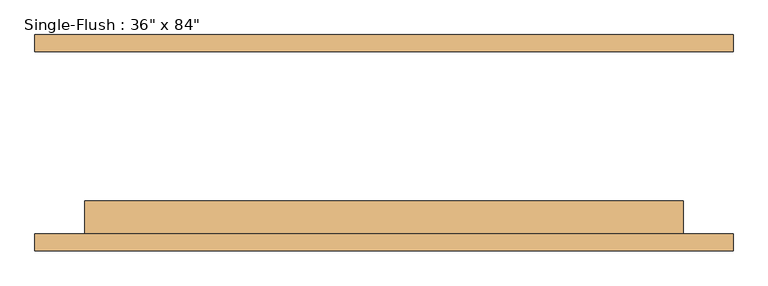
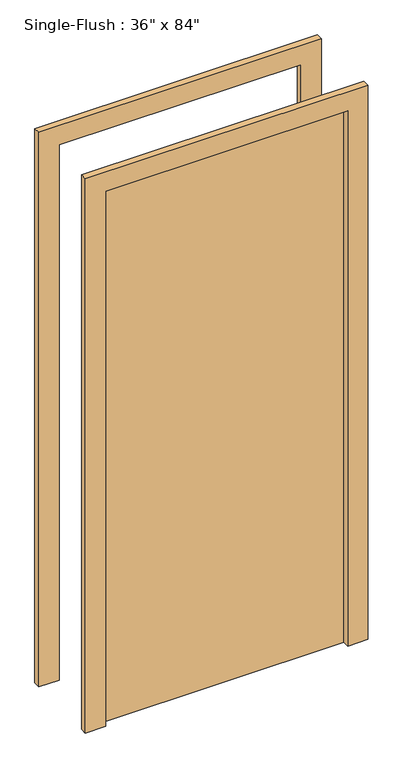
"""IFC4 building model written with IfcOpenShell, lengths in millimetres: door geometry."""

from ifc_helpers import new_model, si_unit, frame, origin, origin_with_axes, place, context, project, spatial, polyline, outline, extrude, source, transform, mapped, element, save


def door_1da80235(model_context):
    return source(origin(), model_context, "Body", "SweptSolid", [
        extrude(outline(polyline([(2209.8, -533.4), (0.0, -533.4), (0.0, -457.2), (2133.6, -457.2), (2133.6, 457.2), (0.0, 457.2), (0.0, 533.4), (2209.8, 533.4), (2209.8, -533.4)])), frame((0.0, -165.1, 0.0), z_axis=(0.0, 1.0, 0.0), x_axis=(0.0, 0.0, 1.0)), (0.0, 0.0, 1.0), 25.4),
        extrude(outline(polyline([(2209.8, 533.4), (2209.8, -533.4), (0.0, -533.4), (0.0, -457.2), (2133.6, -457.2), (2133.6, 457.2), (0.0, 457.2), (0.0, 533.4), (2209.8, 533.4)])), frame((0.0, 139.7, 0.0), z_axis=(0.0, 1.0, 0.0), x_axis=(0.0, 0.0, 1.0)), (0.0, 0.0, 1.0), 25.4),
        extrude(outline(polyline([(457.2, -88.9), (457.2, -139.7), (-457.2, -139.7), (-457.2, -88.9), (457.2, -88.9)])), origin_with_axes(), (0.0, 0.0, 1.0), 2133.6),
    ])


if __name__ == "__main__":
    model = new_model("IFC4")
    model_context = context("Model", 3, world=origin())
    ifc_project = project(units=[si_unit("LENGTHUNIT", "METRE", prefix="MILLI")], contexts=[model_context])
    site = spatial("IfcSite", under=ifc_project)
    building = spatial("IfcBuilding", under=site)
    placement = place(None, origin())
    door_shape = door_1da80235(model_context)
    element("IfcDoor", 1, ObjectType="Single-Flush : 36\" x 84\"", at=placement, inside=building, context=model_context, shape_type="MappedRepresentation", body=[
        mapped(door_shape, transform((0.0, 0.0, 0.0), x_axis=(1.0, 0.0, 0.0), y_axis=(0.0, 1.0, 0.0), z_axis=(0.0, 0.0, 1.0))),
    ])
    save(model, "model.ifc")

# Revit data of these elements
# Type "Single-Flush : 36\" x 84\""
#   Type Mark = "1"
#   Construction Type Id = "MDOOR"
#   Assembly Code = "C1020"
#   Analytic Construction = "Metal"
#   Thickness = 0' - 2"
#   Heat Transfer Coefficient (U) = 0.651978 BTU/(h·ft²·°F)
#   Height = 7' - 0"
#   Trim Projection Ext = 0' - 1"
#   Trim Projection Int = 0' - 1"
#   Trim Width = 0' - 3"
#   Width = 3' - 0"
#   Define Thermal Properties by = 1
#   Define Thermal Properties by = 1
#   Door Material = Door - Panel
#   Frame Material = Door - Frame
#   Visual Light Transmittance = 0
#   Solar Heat Gain Coefficient = 0
#   Function = (empty or 0)
#   Wall Closure = (empty or 0)
# Element 1 (IfcDoor, "Single-Flush : 36\" x 84\"")
#   Materials on its faces: "Door - Frame", "Door - Panel"
# Materials
#   "Door - Panel": class "Wood", colour RGB 210 159 95, transparency 0, Cost = 0
#   "Door - Frame": colour RGB 118 70 51, transparency 0, Cost = 0
